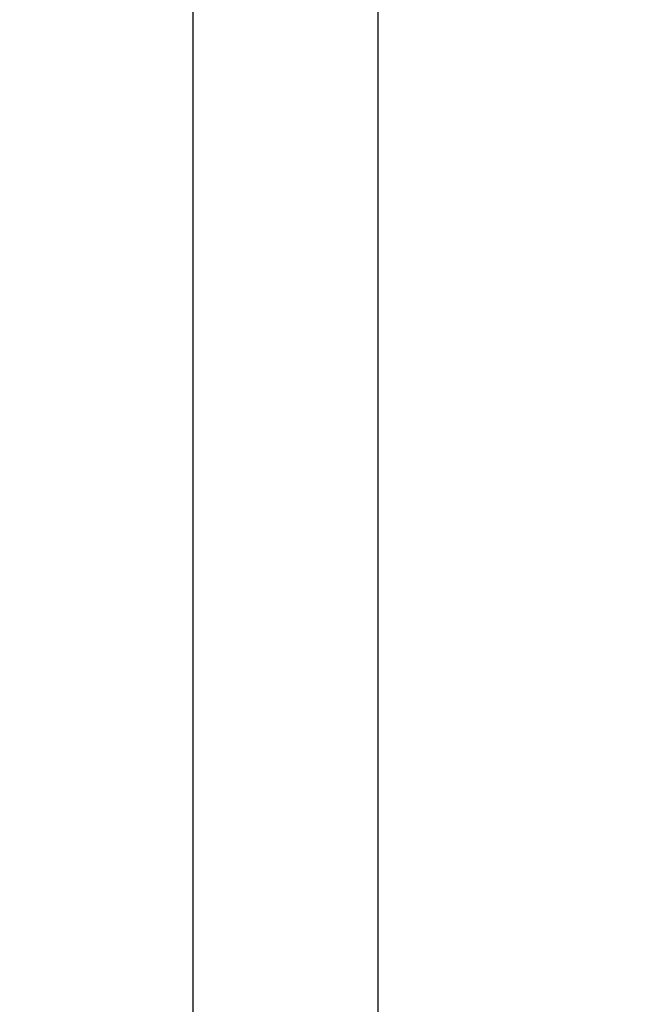
# Model space of a CAD drawing. Units: millimetres. Extents: x 7894 to 8038, y 6851 to 6951.
# Tile 43 of 49: x 7936.33 to 7942.81, y 6931.89 to 6942.2. Entities that reach past the tile are written whole.
import ezdxf

# ---------------------------------------------------------------- set-up
doc = ezdxf.new("R2010")
doc.units = ezdxf.units.MM
doc.layers.add('A-ANNO-DIMS', color=2, linetype='Continuous', lineweight=18)
doc.styles.get("Standard").update_dxf_attribs({"font": 'arial.ttf'})
doc.dimstyles.new('ISO-25', dxfattribs={"dimtxt": 1, "dimasz": 1, "dimexe": 1.25, "dimexo": 0.625, "dimtad": 1, "dimdec": 0, "dimlunit": 4, "dimtxsty": 'Standard', "dimcen": 2.5, "dimclrt": 1, "dimadec": 0, "dimazin": 0, "dimtfac": 1, "dimtdec": 0, "dimtmove": 0, "dimatfit": 3, "dimfxl": 1, "dimarcsym": 0})

# ---------------------------------------------------------------- blocks, each defined once
blk = doc.blocks.new('*D17')
at = {"layer": 'A-ANNO-DIMS', "color": 0, "lineweight": -2, "transparency": 16777216}
for p, q in [((7945.291, 6935.394), (7945.291, 6950.748)), ((7945.192, 6935.394), (7944.041, 6935.394)), ((7945.291, 6932.885), (7945.291, 6934.394)), ((7945.192, 6931.885), (7944.041, 6931.885))]:
    blk.add_line(p, q, dxfattribs=at)
at = {"layer": 'A-ANNO-DIMS', "color": 0, "transparency": 16777216}
for points in [[(7945.124, 6934.394), (7945.457, 6934.394), (7945.291, 6935.394)], [(7945.124, 6932.885), (7945.457, 6932.885), (7945.291, 6931.885)]]:
    blk.add_solid(points, dxfattribs=at)
at = {"layer": 'Defpoints', "color": 0, "transparency": 16777216}
for p in [(7945.291, 6935.394), (7945.817, 6935.394), (7945.817, 6931.885)]:
    blk.add_point(p, dxfattribs=at)
at = {"layer": 'A-ANNO-DIMS', "color": 1, "transparency": 16777216, "insert": (7944.148, 6943.571), "char_height": 1, "attachment_point": 5, "rotation": 90}
blk.add_mtext('FINIAL 0\'-3 1/2" TYP.', dxfattribs=at)
blk = doc.blocks.new('*D23')
at = {"layer": 'A-ANNO-DIMS', "color": 0, "lineweight": -2, "transparency": 16777216}
for p, q in [((7940.089, 6907.098), (7940.089, 6947.793)), ((7971.936, 6928.989), (7971.936, 6947.793)), ((7941.089, 6946.543), (7970.936, 6946.543))]:
    blk.add_line(p, q, dxfattribs=at)
at = {"layer": 'A-ANNO-DIMS', "color": 0, "transparency": 16777216}
for points in [[(7941.089, 6946.709), (7941.089, 6946.376), (7940.089, 6946.543)], [(7970.936, 6946.709), (7970.936, 6946.376), (7971.936, 6946.543)]]:
    blk.add_solid(points, dxfattribs=at)
at = {"layer": 'Defpoints', "color": 0, "transparency": 16777216}
for p in [(7971.936, 6946.543), (7971.936, 6928.364), (7940.089, 6906.473)]:
    blk.add_point(p, dxfattribs=at)
at = {"layer": 'A-ANNO-DIMS', "color": 1, "transparency": 16777216, "insert": (7956.012, 6947.678), "char_height": 1, "attachment_point": 5}
blk.add_mtext('2\'-8"', dxfattribs=at)
blk = doc.blocks.new('*D24')
at = {"layer": 'A-ANNO-DIMS', "color": 0, "lineweight": -2, "transparency": 16777216}
for p, q in [((7953.341, 6944.606), (7936.902, 6944.606)), ((7938.152, 6907.473), (7938.152, 6943.606)), ((7939.464, 6906.473), (7936.902, 6906.473))]:
    blk.add_line(p, q, dxfattribs=at)
at = {"layer": 'A-ANNO-DIMS', "color": 0, "transparency": 16777216}
for points in [[(7937.986, 6943.606), (7938.319, 6943.606), (7938.152, 6944.606)], [(7937.986, 6907.473), (7938.319, 6907.473), (7938.152, 6906.473)]]:
    blk.add_solid(points, dxfattribs=at)
at = {"layer": 'Defpoints', "color": 0, "transparency": 16777216}
for p in [(7938.152, 6944.606), (7953.966, 6944.606), (7940.089, 6906.473)]:
    blk.add_point(p, dxfattribs=at)
at = {"layer": 'A-ANNO-DIMS', "color": 1, "transparency": 16777216, "insert": (7937.016, 6925.539), "char_height": 1, "attachment_point": 5, "rotation": 90}
blk.add_mtext('3\'-2"', dxfattribs=at)
blk = doc.blocks.new('*D35')
at = {"layer": 'A-ANNO-DIMS', "color": 0, "lineweight": -2, "transparency": 16777216}
for p, q in [((7942.957, 6936.255), (7942.957, 6903.287)), ((7943.737, 6929.533), (7943.737, 6903.287)), ((7941.957, 6904.537), (7937.049, 6904.537)), ((7943.737, 6904.537), (7942.957, 6904.537)), ((7944.737, 6904.537), (7945.737, 6904.537))]:
    blk.add_line(p, q, dxfattribs=at)
at = {"layer": 'A-ANNO-DIMS', "color": 0, "transparency": 16777216}
for points in [[(7941.957, 6904.703), (7941.957, 6904.37), (7942.957, 6904.537)], [(7944.737, 6904.703), (7944.737, 6904.37), (7943.737, 6904.537)]]:
    blk.add_solid(points, dxfattribs=at)
at = {"layer": 'Defpoints', "color": 0, "transparency": 16777216}
for p in [(7942.957, 6936.88), (7943.737, 6930.158), (7942.957, 6904.537)]:
    blk.add_point(p, dxfattribs=at)
at = {"layer": 'A-ANNO-DIMS', "color": 1, "transparency": 16777216, "insert": (7939.003, 6905.672), "char_height": 1, "attachment_point": 5}
blk.add_mtext('0\'-1"', dxfattribs=at)

msp = doc.modelspace()

# ---------------------------------------------------------------- dimensions: what is measured, and where the dimension line sits
at = {"layer": 'A-ANNO-DIMS'}
dim = msp.add_linear_dim(base=(7945.291, 6935.394), p1=(7945.817, 6931.885), p2=(7945.817, 6935.394), angle=90, text='FINIAL <> TYP.', dimstyle='ISO-25', override={"dimdec": 1, "dimlfac": 1, "dimrnd": 0, "dimzin": 1, "dimdsep": 46, "dimlunit": 4, "dimfrac": 2}, dxfattribs=at)
dim.commit()
dim.dimension.update_dxf_attribs({"geometry": '*D17', "text_midpoint": (7944.148, 6943.571)})
for base, p1, p2, picture, middle in [((7971.936, 6946.543), (7940.089, 6906.473), (7971.936, 6928.364), '*D23', (7956.012, 6947.678)), ((7942.957, 6904.537), (7943.737, 6930.158), (7942.957, 6936.88), '*D35', (7939.003, 6905.672))]:
    dim = msp.add_linear_dim(base=base, p1=p1, p2=p2, dimstyle='ISO-25', override={"dimdec": 1, "dimlfac": 1, "dimrnd": 0, "dimzin": 1, "dimdsep": 46, "dimlunit": 4, "dimfrac": 2}, dxfattribs=at)
    dim.commit()
    dim.dimension.update_dxf_attribs({"geometry": picture, "text_midpoint": middle})
dim = msp.add_linear_dim(base=(7938.152, 6944.606), p1=(7940.089, 6906.473), p2=(7953.966, 6944.606), angle=90, dimstyle='ISO-25', override={"dimdec": 1, "dimlfac": 1, "dimrnd": 0, "dimzin": 1, "dimdsep": 46, "dimlunit": 4, "dimfrac": 2}, dxfattribs=at)
dim.commit()
dim.dimension.update_dxf_attribs({"geometry": '*D24', "text_midpoint": (7937.016, 6925.539)})

doc.saveas('drawing.dxf')
